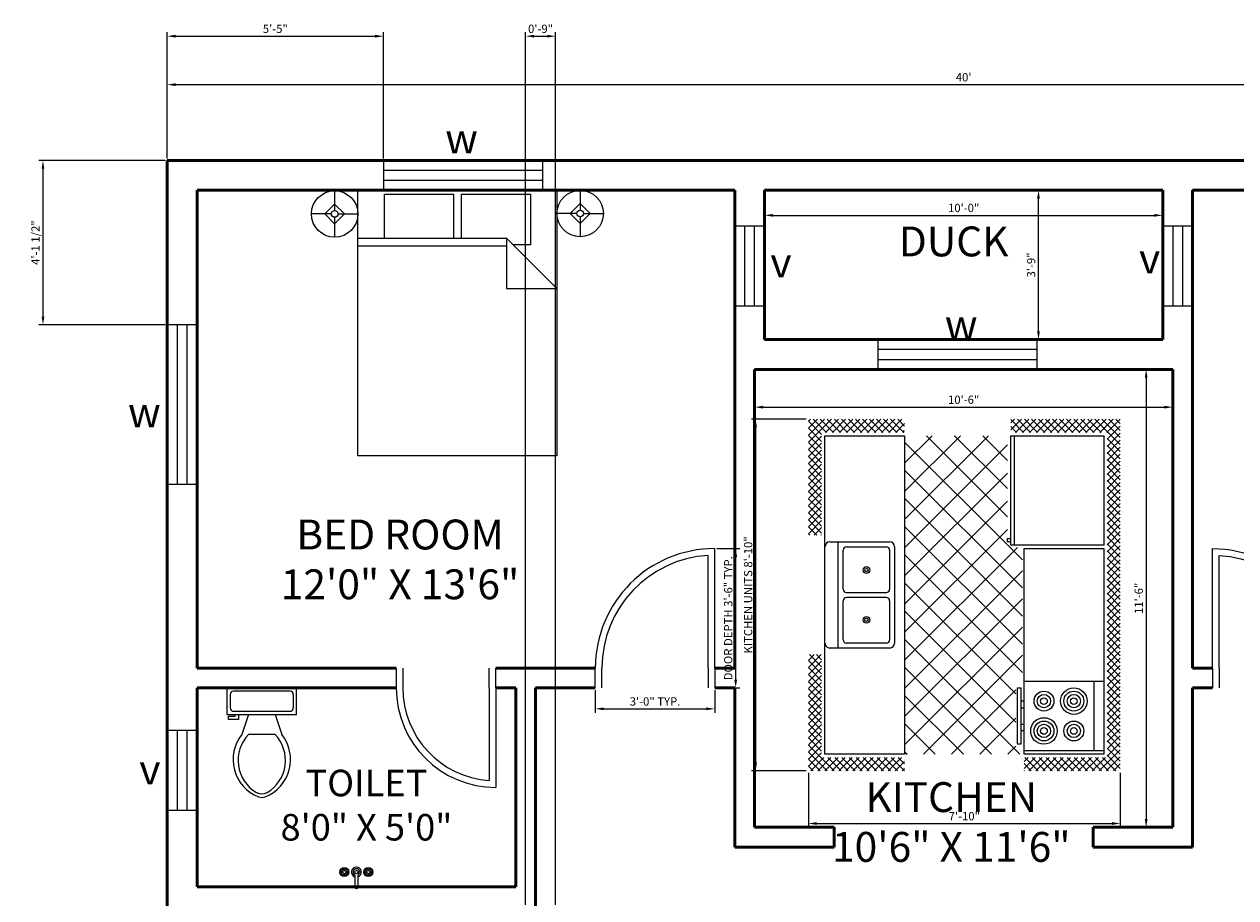
# Model space of a CAD drawing. Units: inches. Extents: x 1776 to 2338, y 1299 to 2099.
# Tile 3 of 4: x 1776 to 2141, y 1836 to 2099. Entities that reach past the tile are written whole.
import ezdxf

# ---------------------------------------------------------------- set-up
doc = ezdxf.new("R2010")
doc.units = ezdxf.units.IN
for name, color, linetype, lineweight in [('A-ANNO-DIMS', 2, 'Continuous', 18), ('A-ANNO-TEXT', 7, 'Continuous', 18), ('A-AREA-IDEN', 7, 'Continuous', 25), ('A-DOOR', 4, 'Continuous', 25), ('A-FLOR-FIXT', 9, 'Continuous', 18), ('A-FURN', 8, 'Continuous', 18), ('A-GLAZ', 4, 'Continuous', 18), ('A-WALL', 7, 'Continuous', 50), ('E-LITE', 9, 'Continuous', 18)]:
    doc.layers.add(name, color=color, linetype=linetype, lineweight=lineweight)
doc.styles.get("Standard").update_dxf_attribs({"font": 'arial.ttf'})
doc.dimstyles.new('ISO-25', dxfattribs={"dimtxt": 2.5, "dimasz": 2.5, "dimexe": 1.25, "dimexo": 0.625, "dimtad": 1, "dimdec": 0, "dimlunit": 3, "dimtxsty": 'Standard', "dimcen": 2.5, "dimadec": 0, "dimazin": 0, "dimtfac": 1, "dimtdec": 0, "dimtmove": 0, "dimatfit": 3, "dimfxl": 1, "dimarcsym": 0})

# ---------------------------------------------------------------- blocks, each defined once
blk = doc.blocks.new('Kitchen Layout - 7 x 8 ft')
for p, q in [((-5, 81.32), (2.68, 89)), ((-5, 83.44), (0.56, 89)), ((-5, 85.56), (-1.56, 89)), ((-5, 87.68), (-3.68, 89)), ((-1, 84.97), (-5, 88.97)), ((1.09, 85), (-2.91, 89)), ((3.21, 85), (-0.79, 89)), ((0.81, 85), (4.81, 89)), ((5.34, 85), (1.34, 89)), ((2.93, 85), (6.93, 89)), ((7.46, 85), (3.46, 89)), ((5.05, 85), (9.05, 89)), ((9.58, 85), (5.58, 89)), ((7.17, 85), (11.17, 89)), ((11.7, 85), (7.7, 89)), ((9.29, 85), (13.29, 89)), ((13.82, 85), (9.82, 89)), ((11.41, 85), (15.41, 89)), ((15.94, 85), (11.94, 89)), ((13.53, 85), (17.53, 89)), ((18.06, 85), (14.06, 89)), ((15.65, 85), (19.65, 89)), ((20.18, 85), (16.18, 89)), ((17.78, 85), (21.78, 89)), ((22.31, 85), (18.31, 89)), ((19.9, 85), (23.9, 89)), ((24.43, 85), (20.43, 89)), ((22.02, 85), (26.02, 89)), ((26.55, 85), (22.55, 89)), ((24.14, 85), (28.14, 89)), ((28.67, 85), (24.67, 89)), ((26.26, 85), (30.26, 89)), ((30.79, 85), (26.79, 89)), ((28.38, 85), (32.38, 89)), ((32.91, 85), (28.91, 89)), ((30.5, 85), (34.5, 89)), ((35.03, 85), (31.03, 89)), ((32.63, 85), (36.63, 89)), ((37.16, 85), (33.16, 89)), ((34.75, 85), (38.75, 89)), ((39.28, 85), (35.28, 89)), ((36.87, 85), (40.87, 89)), ((41.4, 85), (37.4, 89)), ((38.99, 85), (42.99, 89)), ((43.52, 85), (39.52, 89)), ((41.11, 85), (45.11, 89)), ((45.64, 85), (41.64, 89)), ((43.23, 85), (47.23, 89)), ((47.76, 85), (43.76, 89)), ((45.35, 85), (49.35, 89)), ((49.88, 85), (45.88, 89)), ((47.47, 85), (51.47, 89)), ((52, 85), (48, 89)), ((49.6, 85), (53.6, 89)), ((54.13, 85), (50.13, 89)), ((51.72, 85), (55.72, 89)), ((56.25, 85), (52.25, 89)), ((53.84, 85), (57.84, 89)), ((58.37, 85), (54.37, 89)), ((55.96, 85), (59.96, 89)), ((60.49, 85), (56.49, 89)), ((58.08, 85), (62.08, 89)), ((62.61, 85), (58.61, 89)), ((60.2, 85), (64.2, 89)), ((64.73, 85), (60.73, 89)), ((62.32, 85), (66.32, 89)), ((66.85, 85), (62.85, 89)), ((64.45, 85), (68.45, 89)), ((68.97, 85), (64.97, 89)), ((66.57, 85), (70.57, 89)), ((71.1, 85), (67.1, 89)), ((68.69, 85), (72.69, 89)), ((73.22, 85), (69.22, 89)), ((70.81, 85), (74.81, 89)), ((75.34, 85), (71.34, 89)), ((72.93, 85), (76.93, 89)), ((77.46, 85), (73.46, 89)), ((75.05, 85), (79.05, 89)), ((79.58, 85), (75.58, 89)), ((77.17, 85), (81.17, 89)), ((81.7, 85), (77.7, 89)), ((79.29, 85), (83.29, 89)), ((83.82, 85), (79.82, 89)), ((81.42, 85), (85.42, 89)), ((85.95, 85), (81.95, 89)), ((83.54, 85), (87.54, 89)), ((88.07, 85), (84.07, 89)), ((85.66, 85), (89.66, 89)), ((90.19, 85), (86.19, 89)), ((87.78, 85), (91.78, 89)), ((92.31, 85), (88.31, 89)), ((89.9, 85), (93.9, 89)), ((94.43, 85), (90.43, 89)), ((92.02, 85), (96.02, 89)), ((96.55, 85), (92.55, 89)), ((94.14, 85), (98.14, 89)), ((101, 82.67), (94.67, 89)), ((96.27, 85), (100.27, 89)), ((101, 84.79), (96.79, 89)), ((101, 86.92), (98.92, 89)), ((-1, 82.85), (-5, 86.85)), ((-1, 80.73), (-5, 84.73)), ((34, 84), (96, 84)), ((34, 60), (34, 84)), ((96, 84), (96, 60)), ((97, 83.61), (101, 87.61)), ((97, 81.49), (101, 85.49)), ((101, 80.55), (97, 84.55)), ((-5, 79.19), (-1, 83.19)), ((-1, 78.61), (-5, 82.61)), ((-5, 77.07), (-1, 81.07)), ((-1, 76.49), (-5, 80.49)), ((74, 81), (95, 81)), ((97, 79.37), (101, 83.37)), ((101, 78.43), (97, 82.43)), ((97, 77.25), (101, 81.25)), ((-5, 74.95), (-1, 78.95)), ((-1, 74.36), (-5, 78.36)), ((-5, 72.83), (-1, 76.83)), ((101, 76.31), (97, 80.31)), ((97, 75.13), (101, 79.13)), ((101, 74.19), (97, 78.19)), ((97, 73.01), (101, 77.01)), ((-1, 72.24), (-5, 76.24)), ((-5, 70.71), (-1, 74.71)), ((-1, 70.12), (-5, 74.12)), ((101, 72.07), (97, 76.07)), ((97, 70.89), (101, 74.89)), ((101, 69.95), (97, 73.95)), ((-5, 68.59), (-1, 72.59)), ((-1, 68), (-5, 72)), ((-5, 66.47), (-1, 70.47)), ((-1, 65.88), (-5, 69.88)), ((97, 68.76), (101, 72.76)), ((101, 67.82), (97, 71.82)), ((97, 66.64), (101, 70.64)), ((101, 65.7), (97, 69.7)), ((-5, 64.35), (-1, 68.35)), ((-1, 63.76), (-5, 67.76)), ((-5, 62.22), (-1, 66.22)), ((97, 64.52), (101, 68.52)), ((101, 63.58), (97, 67.58)), ((97, 62.4), (101, 66.4)), ((-1, 61.64), (-5, 65.64)), ((-5, 60.1), (-1, 64.1)), ((-1, 59.52), (-5, 63.52)), ((101, 61.46), (97, 65.46)), ((97, 60.28), (101, 64.28)), ((100.34, 60), (97, 63.34)), ((98.84, 60), (101, 62.16)), ((-5, 57.98), (-1, 61.98)), ((-1, 57.39), (-5, 61.39)), ((-1.73, 56), (-5, 59.27)), ((-4.86, 56), (-1, 59.86)), ((10.4, 24), (45.9, 59.5)), ((18.88, 24), (54.38, 59.5)), ((27.37, 24), (62.87, 59.5)), ((33.03, 55.11), (37.41, 59.5)), ((96, 60), (34, 60)), ((35.85, 24), (71.35, 59.5)), ((76.2, 24), (40.7, 59.5)), ((84.68, 24), (49.18, 59.5)), ((93.17, 24), (57.67, 59.5)), ((61.31, 24), (96, 58.69)), ((96, 29.65), (66.15, 59.5)), ((80, 60), (80, 59)), ((82, 59), (82, 60)), ((87, 59), (87, 60)), ((89, 60), (89, 59)), ((98.22, 60), (97, 61.22)), ((100.96, 60), (101, 60.04)), ((-3.85, 56), (-5, 57.15)), ((-2.74, 56), (-1, 57.74)), ((0, 57), (33, 57)), ((0, 30.57), (24.43, 55)), ((0, 39.06), (15.94, 55)), ((0, 47.54), (7.46, 55)), ((1.91, 24), (32.91, 55)), ((33.77, 24), (2.77, 55)), ((42.26, 24), (11.26, 55)), ((50.74, 24), (19.74, 55)), ((59.23, 24), (28.23, 55)), ((31, 55), (31, 56)), ((32, 55), (31, 55)), ((32, 56), (32, 55)), ((67.71, 24), (33.68, 58.04)), ((44.34, 24), (77.84, 57.5)), ((52.82, 24), (86.32, 57.5)), ((96, 38.14), (76.64, 57.5)), ((96, 46.63), (85.13, 57.5)), ((96, 55.11), (93.57, 57.54)), ((25.29, 24), (0, 49.29)), ((69.79, 24), (96, 50.21)), ((16.8, 24), (0, 40.8)), ((78.28, 24), (96, 41.72)), ((86.76, 24), (96, 33.24)), ((8.32, 24), (0, 32.32)), ((-5, 21.92), (-2.92, 24)), ((-5, 19.8), (-1, 23.8)), ((-1, 19.21), (-5, 23.21)), ((-1, 21.33), (-3.67, 24)), ((-1, 23.45), (-1.55, 24)), ((0, 24), (96, 24)), ((0, 0), (0, 24)), ((95.25, 24), (96, 24.75)), ((96, 24), (96, 0)), ((97, 22.1), (98.9, 24)), ((97, 19.97), (101, 23.97)), ((101, 19.03), (97, 23.03)), ((101, 21.16), (98.16, 24)), ((101, 23.28), (100.28, 24)), ((-5, 17.68), (-1, 21.68)), ((-1, 17.09), (-5, 21.09)), ((-5, 15.55), (-1, 19.55)), ((-1, 14.97), (-5, 18.97)), ((47.25, 6.5), (47.25, 18.5)), ((48.75, 18.5), (48.75, 6.5)), ((97, 17.85), (101, 21.85)), ((101, 16.91), (97, 20.91)), ((97, 15.73), (101, 19.73)), ((101, 14.79), (97, 18.79)), ((-5, 13.43), (-1, 17.43)), ((-1, 12.85), (-5, 16.85)), ((-5, 11.31), (-1, 15.31)), ((-1, 10.73), (-5, 14.73)), ((97, 13.61), (101, 17.61)), ((101, 12.67), (97, 16.67)), ((97, 11.49), (101, 15.49)), ((-5, 9.19), (-1, 13.19)), ((-1, 8.6), (-5, 12.6)), ((-5, 7.07), (-1, 11.07)), ((101, 10.55), (97, 14.55)), ((97, 9.37), (101, 13.37)), ((101, 8.43), (97, 12.43)), ((97, 7.25), (101, 11.25)), ((-1, 6.48), (-5, 10.48)), ((-5, 4.95), (-1, 8.95)), ((-1, 4.36), (-5, 8.36)), ((101, 6.31), (97, 10.31)), ((97, 5.12), (101, 9.12)), ((101, 4.18), (97, 8.18)), ((-5, 2.83), (-1, 6.83)), ((-1, 2.24), (-5, 6.24)), ((-5, 0.71), (-1, 4.71)), ((-1, 0.12), (-5, 4.12)), ((64, 4), (32, 4)), ((97, 3), (101, 7)), ((101, 2.06), (97, 6.06)), ((97, 0.88), (101, 4.88)), ((101, -0.06), (97, 3.94)), ((-5, -1.42), (-1, 2.58)), ((2, -5), (-5, 2)), ((-5, -3.54), (-1, 0.46)), ((96, 0), (0, 0)), ((93.24, -5), (101, 2.76)), ((95.36, -5), (101, 0.64)), ((101, -2.18), (97, 1.82)), ((-0.12, -5), (-5, -0.12)), ((-2.25, -5), (-5, -2.25)), ((-4.34, -5), (-0.34, -1)), ((-2.22, -5), (1.78, -1)), ((-0.1, -5), (3.9, -1)), ((4.12, -5), (0.12, -1)), ((2.02, -5), (6.02, -1)), ((6.24, -5), (2.24, -1)), ((4.14, -5), (8.14, -1)), ((8.36, -5), (4.36, -1)), ((6.27, -5), (10.27, -1)), ((10.48, -5), (6.48, -1)), ((8.39, -5), (12.39, -1)), ((12.6, -5), (8.6, -1)), ((10.51, -5), (14.51, -1)), ((14.73, -5), (10.73, -1)), ((12.63, -5), (16.63, -1)), ((16.85, -5), (12.85, -1)), ((14.75, -5), (18.75, -1)), ((18.97, -5), (14.97, -1)), ((16.87, -5), (20.87, -1)), ((21.09, -5), (17.09, -1)), ((18.99, -5), (22.99, -1)), ((23.21, -5), (19.21, -1)), ((21.11, -5), (25.11, -1)), ((25.33, -5), (21.33, -1)), ((23.24, -5), (27.24, -1)), ((27.45, -5), (23.45, -1)), ((25.36, -5), (29.36, -1)), ((29.57, -5), (25.57, -1)), ((27.48, -5), (30, -2.48)), ((30, -3.3), (27.7, -1)), ((30, -1.18), (29.82, -1)), ((66, -2.54), (67.54, -1)), ((66, -4.66), (69.66, -1)), ((69.88, -5), (66, -1.12)), ((67.76, -5), (66, -3.24)), ((67.78, -5), (71.78, -1)), ((72, -5), (68, -1)), ((69.9, -5), (73.9, -1)), ((74.12, -5), (70.12, -1)), ((72.03, -5), (76.03, -1)), ((76.24, -5), (72.24, -1)), ((74.15, -5), (78.15, -1)), ((78.36, -5), (74.36, -1)), ((76.27, -5), (80.27, -1)), ((80.49, -5), (76.49, -1)), ((78.39, -5), (82.39, -1)), ((82.61, -5), (78.61, -1)), ((80.51, -5), (84.51, -1)), ((84.73, -5), (80.73, -1)), ((82.63, -5), (86.63, -1)), ((86.85, -5), (82.85, -1)), ((84.75, -5), (88.75, -1)), ((88.97, -5), (84.97, -1)), ((86.88, -5), (90.88, -1)), ((91.09, -5), (87.09, -1)), ((89, -5), (93, -1)), ((93.21, -5), (89.21, -1)), ((91.12, -5), (95.12, -1)), ((95.34, -5), (91.34, -1)), ((97.46, -5), (93.46, -1)), ((99.58, -5), (95.58, -1)), ((101, -4.3), (97, -0.3)), ((97.48, -5), (101, -1.48)), ((99.6, -5), (101, -3.6)), ((-4.37, -5), (-5, -4.37)), ((29.6, -5), (30, -4.6))]:
    blk.add_line(p, q)
for points in [[(0, 56), (0, 84), (33, 84), (33, 56)], [(74, 60), (74, 84), (95, 84), (95, 60)], [(76, 58), (76, 59), (93, 59), (93, 58)]]:
    blk.add_lwpolyline(points, close=True)
for points in [[(32, 1.5), (32, 19.5)], [(33.5, 21), (62.5, 21)], [(33.5, 6.5), (33.5, 18.5)], [(34.5, 19.5), (46.25, 19.5)], [(49.75, 19.5), (61.5, 19.5)], [(62.5, 18.5), (62.5, 6.5)], [(64, 19.5), (64, 1.5)], [(46.25, 5.5), (34.5, 5.5)], [(61.5, 5.5), (49.75, 5.5)], [(62.5, 0), (33.5, 0)]]:
    blk.add_lwpolyline(points)
for centre, radius in [((80, 75), 4), ((80, 75), 3), ((80, 75), 2), ((89, 75), 3), ((89, 75), 2), ((80, 75), 1), ((89, 75), 1), ((89, 66), 4), ((80, 66), 3), ((80, 66), 2), ((80, 66), 1), ((89, 66), 3), ((89, 66), 2), ((89, 66), 1), ((40.5, 12.5), 1), ((40.5, 12.5), 0.5), ((55.5, 12.5), 1), ((55.5, 12.5), 0.5)]:
    blk.add_circle(centre, radius)
for centre, radius, start, end in [((33.5, 19.5), 1.5, 90, 180), ((34.5, 18.5), 1, 90, 180), ((46.25, 18.5), 1, 0, 90), ((49.75, 18.5), 1, 90, 180), ((61.5, 18.5), 1, 0, 90), ((62.5, 19.5), 1.5, 0, 90), ((34.5, 6.5), 1, 180, 270), ((46.25, 6.5), 1, 270, 0), ((49.75, 6.5), 1, 180, 270), ((61.5, 6.5), 1, 270, 0), ((33.5, 1.5), 1.5, 180, 270), ((62.5, 1.5), 1.5, 270, 0)]:
    blk.add_arc(centre, radius, start, end)
blk = doc.blocks.new('Bed - Queen')
for p, q in [((0, -80.00003), (0, 0)), ((0, 0), (59.99999, 0)), ((59.99999, 0), (59.99999, -80.00003)), ((7.99999, -1.2), (28.79998, -1.2)), ((7.99999, -14.4), (7.99999, -1.2)), ((28.79998, -1.2), (28.79998, -14.4)), ((31.19999, -1.2), (51.99999, -1.2)), ((31.19999, -14.4), (31.19999, -1.2)), ((51.99999, -1.2), (51.99999, -16.4)), ((0, -14.4), (44.8, -14.4)), ((59.99999, -29.6), (44.8, -14.4)), ((44.8, -14.4), (44.8, -29.6)), ((44.8, -16.8), (0, -16.8)), ((51.99999, -16.4), (46.79936, -16.4)), ((44.8, -29.6), (59.99999, -29.6)), ((59.99999, -80.00003), (0, -80.00003))]:
    blk.add_line(p, q)
blk = doc.blocks.new('Lamp - Table')
for p, q in [((0, 7), (0, 1)), ((-1, 0), (-7, 0)), ((0, 3), (-3, 0)), ((-3, 0), (0, -3)), ((3, 0), (0, 3)), ((0, -3), (3, 0)), ((1, 0), (7, 0)), ((0, -1), (0, -7))]:
    blk.add_line(p, q)
for radius in [7, 1]:
    blk.add_circle((0, 0), radius)
blk = doc.blocks.new('Toilet - top')
for p, q in [((9.5, -6), (9.5, -2)), ((-10, -8.5), (-8, -8.5)), ((-10, -9.5), (-10, -8.5)), ((-7, -9.5), (-10, -9.5)), ((-8, -8.5), (-8, -8)), ((-7, -8), (-7, -9.5)), ((-4, -8), (-6, -14)), ((4, -8), (6, -14)), ((4, -14), (-4, -14))]:
    blk.add_line(p, q)
blk.add_lwpolyline([(10.5, -8), (10.5, 0), (-10.5, 0), (-10.5, -8)], close=True)
for points in [[(-9.5, -2), (-9.5, -6)], [(8.5, -1), (-8.5, -1)], [(-8.5, -7), (8.5, -7)]]:
    blk.add_lwpolyline(points)
for centre, radius, start, end in [((-8.62, -1.88), 0.884, 81.8699, 188.1301), ((8.62, -1.88), 0.884, 351.8699, 98.1301), ((-8.62, -6.12), 0.884, 171.8699, 278.1301), ((8.62, -6.12), 0.884, 261.8699, 8.1301), ((3.52, -21.58), 12.17, 141.4691, 247.9714), ((4.2, -21.82), 11.33, 136.3677, 238.9468), ((-3.52, -21.58), 12.17, 292.0284, 38.5307), ((-4.2, -21.82), 11.33, 301.053, 43.6321), ((0, -27.88), 4, 245.7318, 294.2682), ((0, -29), 4, 254.8605, 285.1395)]:
    blk.add_arc(centre, radius, start, end)
blk = doc.blocks.new('Faucet - Bathroom top')
for p, q in [((-4.107, 0.125), (-4.375, 0.125)), ((-3.75, 0.4788), (-3.75, 0.75)), ((-3.5, 0.482), (-3.5, 0.75)), ((-3.1461, 0.125), (-2.875, 0.125)), ((3.143, 0.125), (2.875, 0.125)), ((3.5, 0.4788), (3.5, 0.75)), ((3.75, 0.482), (3.75, 0.75)), ((4.1039, 0.125), (4.375, 0.125)), ((-4.1039, -0.125), (-4.375, -0.125)), ((-3.75, -0.4821), (-3.75, -0.75)), ((-3.5, -0.4789), (-3.5, -0.75)), ((-3.143, -0.125), (-2.875, -0.125)), ((-0.5, -0.8639), (-0.5, -4.5)), ((0.5, -4.5), (0.5, -0.8631)), ((3.1461, -0.125), (2.875, -0.125)), ((3.5, -0.4821), (3.5, -0.75)), ((3.75, -0.4789), (3.75, -0.75)), ((4.107, -0.125), (4.375, -0.125))]:
    blk.add_line(p, q)
for centre, radius in [((-3.625, 0), 1.375), ((-4.625, 0), 0.2795), ((-3.625, 0), 0.5), ((-3.625, 1), 0.2795), ((-2.625, 0), 0.2795), ((0, 0), 0.5), ((3.625, 0), 1.375), ((2.625, 0), 0.2795), ((3.625, 0), 0.5), ((3.625, 1), 0.2795), ((4.625, 0), 0.2795), ((-3.625, -1), 0.2795), ((3.625, -1), 0.2795)]:
    blk.add_circle(centre, radius)
for centre, radius, start, end in [((-3.625, 0), 1, 105.2407, 164.2093), ((-3.625, 0), 1, 16.44125, 74.07887), ((0, 0), 1.5, 289.6514, 250.3603), ((0, 0), 1, 300.3431, 239.7554), ((3.625, 0), 1, 106.12, 164.0884), ((3.625, 0), 1, 16.23422, 73.90469), ((-3.625, 0), 1, 196.2342, 253.9047), ((-3.625, 0), 1, 286.12, 344.0884), ((3.625, 0), 1, 196.4413, 254.0789), ((3.625, 0), 1, 285.2407, 344.2093), ((0, -4.5), 0.5, 180, 0)]:
    blk.add_arc(centre, radius, start, end)
blk = doc.blocks.new('*D9')
at = {"layer": 'A-ANNO-DIMS', "color": 0, "lineweight": -2, "transparency": 16777216}
for p, q in [((1995.74, 1994.59), (1995.74, 1982.6)), ((2121.74, 1994.59), (2121.74, 1982.6)), ((1998.24, 1983.85), (2119.24, 1983.85))]:
    blk.add_line(p, q, dxfattribs=at)
at = {"layer": 'A-ANNO-DIMS', "color": 0, "transparency": 16777216}
for points in [[(1998.24, 1984.27), (1998.24, 1983.44), (1995.74, 1983.85)], [(2119.24, 1984.27), (2119.24, 1983.44), (2121.74, 1983.85)]]:
    blk.add_solid(points, dxfattribs=at)
at = {"layer": 'Defpoints', "color": 0, "transparency": 16777216}
for p in [(1995.74, 1995.22), (2121.74, 1995.22), (2121.74, 1983.85)]:
    blk.add_point(p, dxfattribs=at)
at = {"layer": 'A-ANNO-DIMS', "color": 0, "transparency": 16777216, "insert": (2058.74, 1985.76), "char_height": 2.5, "attachment_point": 5}
blk.add_mtext('10\'-6"', dxfattribs=at)
blk = doc.blocks.new('*D10')
at = {"layer": 'A-ANNO-DIMS', "color": 0, "lineweight": -2, "transparency": 16777216}
for p, q in [((2121.11, 1995.22), (2112.49, 1995.22)), ((2113.74, 1992.72), (2113.74, 1859.72)), ((2121.11, 1857.22), (2112.49, 1857.22))]:
    blk.add_line(p, q, dxfattribs=at)
at = {"layer": 'A-ANNO-DIMS', "color": 0, "transparency": 16777216}
for points in [[(2113.32, 1992.72), (2114.15, 1992.72), (2113.74, 1995.22)], [(2113.32, 1859.72), (2114.15, 1859.72), (2113.74, 1857.22)]]:
    blk.add_solid(points, dxfattribs=at)
at = {"layer": 'Defpoints', "color": 0, "transparency": 16777216}
for p in [(2121.74, 1995.22), (2113.74, 1857.22), (2121.74, 1857.22)]:
    blk.add_point(p, dxfattribs=at)
at = {"layer": 'A-ANNO-DIMS', "color": 0, "transparency": 16777216, "insert": (2111.83, 1926.22), "char_height": 2.5, "attachment_point": 5, "rotation": 90}
blk.add_mtext('11\'-6"', dxfattribs=at)
blk = doc.blocks.new('*D12')
at = {"layer": 'A-ANNO-DIMS', "color": 0, "lineweight": -2, "transparency": 16777216}
for p, q in [((1818.74, 2058.84), (1818.74, 2082.32)), ((1821.24, 2081.07), (2296.24, 2081.07)), ((2298.74, 2058.84), (2298.74, 2082.32))]:
    blk.add_line(p, q, dxfattribs=at)
at = {"layer": 'A-ANNO-DIMS', "color": 0, "transparency": 16777216}
for points in [[(1821.24, 2081.49), (1821.24, 2080.65), (1818.74, 2081.07)], [(2296.24, 2081.49), (2296.24, 2080.65), (2298.74, 2081.07)]]:
    blk.add_solid(points, dxfattribs=at)
at = {"layer": 'Defpoints', "color": 0, "transparency": 16777216}
for p in [(2298.74, 2081.07), (1818.74, 2058.22), (2298.74, 2058.22)]:
    blk.add_point(p, dxfattribs=at)
at = {"layer": 'A-ANNO-DIMS', "color": 0, "transparency": 16777216, "insert": (2058.74, 2082.97), "char_height": 2.5, "attachment_point": 5}
blk.add_mtext("40'", dxfattribs=at)
blk = doc.blocks.new('WIN-48IN')
for p, q in [((48, 9), (0, 9)), ((0, 9), (0, 0)), ((48, 0), (48, 9)), ((48, 6), (0, 6)), ((0, 3), (48, 3)), ((0, 0), (48, 0))]:
    blk.add_line(p, q)
blk = doc.blocks.new('VENT-24IN')
for p, q in [((9, 24), (0, 24)), ((0, 24), (0, 0)), ((3, 24), (3, 0)), ((6, 0), (6, 24)), ((9, 0), (9, 24)), ((0, 0), (9, 0))]:
    blk.add_line(p, q)
blk = doc.blocks.new('DOOR-36IN')
for p, q in [((36, 6), (36, 42)), ((34, 6), (34, 39.94)), ((0, 0), (0, 6)), ((2, 0), (2, 6)), ((34, 6), (34, 0)), ((36, 6), (36, 0))]:
    blk.add_line(p, q)
for radius, start in [(36, 90), (34, 93.3723)]:
    blk.add_arc((36, 6), radius, start, 180)
blk = doc.blocks.new('DOOR-30IN')
for p, q in [((0, 36), (0, 30)), ((2, 36), (2, 30)), ((28, 30), (28, 36)), ((30, 30), (30, 36)), ((28, 30), (28, 2.07)), ((30, 30), (30, 0))]:
    blk.add_line(p, q)
for radius, end in [(30, 270), (28, 265.904)]:
    blk.add_arc((30, 30), radius, 180, end)
blk = doc.blocks.new('*D30')
at = {"layer": 'A-ANNO-DIMS', "color": 0, "lineweight": -2, "transparency": 16777216}
for p, q in [((1984.36, 1941.22), (1991.29, 1941.22)), ((1990.04, 1901.72), (1990.04, 1938.72)), ((1984.36, 1899.22), (1991.29, 1899.22))]:
    blk.add_line(p, q, dxfattribs=at)
at = {"layer": 'A-ANNO-DIMS', "color": 0, "transparency": 16777216}
for points in [[(1989.62, 1938.72), (1990.46, 1938.72), (1990.04, 1941.22)], [(1989.62, 1901.72), (1990.46, 1901.72), (1990.04, 1899.22)]]:
    blk.add_solid(points, dxfattribs=at)
at = {"layer": 'Defpoints', "color": 0, "transparency": 16777216}
for p in [(1983.74, 1941.22), (1990.04, 1941.22), (1983.74, 1899.22)]:
    blk.add_point(p, dxfattribs=at)
at = {"layer": 'A-ANNO-DIMS', "color": 0, "transparency": 16777216, "insert": (1988.12, 1920.22), "char_height": 2.5, "attachment_point": 5, "rotation": 90}
blk.add_mtext('DOOR DEPTH 3\'-6" TYP.', dxfattribs=at)
blk = doc.blocks.new('*D31')
at = {"layer": 'A-ANNO-DIMS', "color": 0, "lineweight": -2, "transparency": 16777216}
for p, q in [((1947.74, 1898.59), (1947.74, 1891.67)), ((1983.74, 1898.59), (1983.74, 1891.67)), ((1950.24, 1892.92), (1981.24, 1892.92))]:
    blk.add_line(p, q, dxfattribs=at)
at = {"layer": 'A-ANNO-DIMS', "color": 0, "transparency": 16777216}
for points in [[(1950.24, 1893.34), (1950.24, 1892.5), (1947.74, 1892.92)], [(1981.24, 1893.34), (1981.24, 1892.5), (1983.74, 1892.92)]]:
    blk.add_solid(points, dxfattribs=at)
at = {"layer": 'Defpoints', "color": 0, "transparency": 16777216}
for p in [(1947.74, 1899.22), (1983.74, 1899.22), (1983.74, 1892.92)]:
    blk.add_point(p, dxfattribs=at)
at = {"layer": 'A-ANNO-DIMS', "color": 0, "transparency": 16777216, "insert": (1965.74, 1894.82), "char_height": 2.5, "attachment_point": 5}
blk.add_mtext('3\'-0" TYP.', dxfattribs=at)
blk = doc.blocks.new('*D40')
at = {"layer": 'A-ANNO-DIMS', "color": 0, "lineweight": -2, "transparency": 16777216}
for p, q in [((2011.31, 1980.25), (1994.79, 1980.25)), ((1996.04, 1977.75), (1996.04, 1876.75)), ((2011.31, 1874.25), (1994.79, 1874.25))]:
    blk.add_line(p, q, dxfattribs=at)
at = {"layer": 'A-ANNO-DIMS', "color": 0, "transparency": 16777216}
for points in [[(1995.62, 1977.75), (1996.45, 1977.75), (1996.04, 1980.25)], [(1995.62, 1876.75), (1996.45, 1876.75), (1996.04, 1874.25)]]:
    blk.add_solid(points, dxfattribs=at)
at = {"layer": 'Defpoints', "color": 0, "transparency": 16777216}
for p in [(2011.94, 1980.25), (1996.04, 1874.25), (2011.94, 1874.25)]:
    blk.add_point(p, dxfattribs=at)
at = {"layer": 'A-ANNO-DIMS', "color": 0, "transparency": 16777216, "insert": (1994.12, 1927.25), "char_height": 2.5, "attachment_point": 5, "rotation": 90}
blk.add_mtext('KITCHEN UNITS 8\'-10"', dxfattribs=at)
blk = doc.blocks.new('*D41')
at = {"layer": 'A-ANNO-DIMS', "color": 0, "lineweight": -2, "transparency": 16777216}
for p, q in [((2011.94, 1873.62), (2011.94, 1857.1)), ((2105.94, 1873.62), (2105.94, 1857.1)), ((2014.44, 1858.35), (2103.44, 1858.35))]:
    blk.add_line(p, q, dxfattribs=at)
at = {"layer": 'A-ANNO-DIMS', "color": 0, "transparency": 16777216}
for points in [[(2014.44, 1858.77), (2014.44, 1857.93), (2011.94, 1858.35)], [(2103.44, 1858.77), (2103.44, 1857.93), (2105.94, 1858.35)]]:
    blk.add_solid(points, dxfattribs=at)
at = {"layer": 'Defpoints', "color": 0, "transparency": 16777216}
for p in [(2011.94, 1874.25), (2105.94, 1874.25), (2105.94, 1858.35)]:
    blk.add_point(p, dxfattribs=at)
at = {"layer": 'A-ANNO-DIMS', "color": 0, "transparency": 16777216, "insert": (2058.94, 1860.25), "char_height": 2.5, "attachment_point": 5}
blk.add_mtext('7\'-10"', dxfattribs=at)
blk = doc.blocks.new('*D45')
at = {"layer": 'A-ANNO-DIMS', "color": 0, "lineweight": -2, "transparency": 16777216}
for p, q in [((1998.74, 2004.84), (1998.74, 2042.92)), ((2001.24, 2041.67), (2116.24, 2041.67)), ((2118.74, 2004.84), (2118.74, 2042.92))]:
    blk.add_line(p, q, dxfattribs=at)
at = {"layer": 'A-ANNO-DIMS', "color": 0, "transparency": 16777216}
for points in [[(2001.24, 2042.09), (2001.24, 2041.25), (1998.74, 2041.67)], [(2116.24, 2042.09), (2116.24, 2041.25), (2118.74, 2041.67)]]:
    blk.add_solid(points, dxfattribs=at)
at = {"layer": 'Defpoints', "color": 0, "transparency": 16777216}
for p in [(2118.74, 2041.67), (1998.74, 2004.22), (2118.74, 2004.22)]:
    blk.add_point(p, dxfattribs=at)
at = {"layer": 'A-ANNO-DIMS', "color": 0, "transparency": 16777216, "insert": (2058.74, 2043.57), "char_height": 2.5, "attachment_point": 5}
blk.add_mtext('10\'-0"', dxfattribs=at)
blk = doc.blocks.new('*D46')
at = {"layer": 'A-ANNO-DIMS', "color": 0, "lineweight": -2, "transparency": 16777216}
for p, q in [((2118.11, 2049.22), (2080.04, 2049.22)), ((2081.29, 2006.72), (2081.29, 2046.72)), ((2118.11, 2004.22), (2080.04, 2004.22))]:
    blk.add_line(p, q, dxfattribs=at)
at = {"layer": 'A-ANNO-DIMS', "color": 0, "transparency": 16777216}
for points in [[(2080.87, 2046.72), (2081.71, 2046.72), (2081.29, 2049.22)], [(2080.87, 2006.72), (2081.71, 2006.72), (2081.29, 2004.22)]]:
    blk.add_solid(points, dxfattribs=at)
at = {"layer": 'Defpoints', "color": 0, "transparency": 16777216}
for p in [(2081.29, 2049.22), (2118.74, 2049.22), (2118.74, 2004.22)]:
    blk.add_point(p, dxfattribs=at)
at = {"layer": 'A-ANNO-DIMS', "color": 0, "transparency": 16777216, "insert": (2079.39, 2026.72), "char_height": 2.5, "attachment_point": 5, "rotation": 90}
blk.add_mtext('3\'-9"', dxfattribs=at)
blk = doc.blocks.new('*D49')
at = {"layer": 'A-ANNO-DIMS', "color": 0, "lineweight": -2, "transparency": 16777216}
for p, q in [((1926.74, 1833.84), (1926.74, 2096.92)), ((1929.24, 2095.67), (1933.24, 2095.67)), ((1935.74, 1833.84), (1935.74, 2096.92))]:
    blk.add_line(p, q, dxfattribs=at)
at = {"layer": 'A-ANNO-DIMS', "color": 0, "transparency": 16777216}
for points in [[(1929.24, 2096.09), (1929.24, 2095.25), (1926.74, 2095.67)], [(1933.24, 2096.09), (1933.24, 2095.25), (1935.74, 2095.67)]]:
    blk.add_solid(points, dxfattribs=at)
at = {"layer": 'Defpoints', "color": 0, "transparency": 16777216}
for p in [(1935.74, 2095.67), (1926.74, 1833.22), (1935.74, 1833.22)]:
    blk.add_point(p, dxfattribs=at)
at = {"layer": 'A-ANNO-DIMS', "color": 0, "transparency": 16777216, "insert": (1931.24, 2097.57), "char_height": 2.5, "attachment_point": 5}
blk.add_mtext('0\'-9"', dxfattribs=at)
blk = doc.blocks.new('*D51')
at = {"layer": 'A-ANNO-DIMS', "color": 0, "lineweight": -2, "transparency": 16777216}
for p, q in [((1818.74, 2058.84), (1818.74, 2096.92)), ((1821.24, 2095.67), (1881.39, 2095.67)), ((1883.89, 2058.84), (1883.89, 2096.92))]:
    blk.add_line(p, q, dxfattribs=at)
at = {"layer": 'A-ANNO-DIMS', "color": 0, "transparency": 16777216}
for points in [[(1821.24, 2096.09), (1821.24, 2095.25), (1818.74, 2095.67)], [(1881.39, 2096.09), (1881.39, 2095.25), (1883.89, 2095.67)]]:
    blk.add_solid(points, dxfattribs=at)
at = {"layer": 'Defpoints', "color": 0, "transparency": 16777216}
for p in [(1883.89, 2095.67), (1818.74, 2058.22), (1883.89, 2058.22)]:
    blk.add_point(p, dxfattribs=at)
at = {"layer": 'A-ANNO-DIMS', "color": 0, "transparency": 16777216, "insert": (1851.31, 2097.57), "char_height": 2.5, "attachment_point": 5}
blk.add_mtext('5\'-5"', dxfattribs=at)
blk = doc.blocks.new('*D53')
at = {"layer": 'A-ANNO-DIMS', "color": 0, "lineweight": -2, "transparency": 16777216}
for p, q in [((1818.11, 2058.22), (1780.04, 2058.22)), ((1781.29, 2055.72), (1781.29, 2011.17)), ((1818.11, 2008.67), (1780.04, 2008.67))]:
    blk.add_line(p, q, dxfattribs=at)
at = {"layer": 'A-ANNO-DIMS', "color": 0, "transparency": 16777216}
for points in [[(1780.87, 2055.72), (1781.71, 2055.72), (1781.29, 2058.22)], [(1780.87, 2011.17), (1781.71, 2011.17), (1781.29, 2008.67)]]:
    blk.add_solid(points, dxfattribs=at)
at = {"layer": 'Defpoints', "color": 0, "transparency": 16777216}
for p in [(1818.74, 2058.22), (1781.29, 2008.67), (1818.74, 2008.67)]:
    blk.add_point(p, dxfattribs=at)
at = {"layer": 'A-ANNO-DIMS', "color": 0, "transparency": 16777216, "insert": (1779.37, 2033.45), "char_height": 2.5, "attachment_point": 5, "rotation": 90}
blk.add_mtext('4\'-1 1/2"', dxfattribs=at)

msp = doc.modelspace()

# ---------------------------------------------------------------- linework, layer by layer
at = {"layer": 'A-WALL'}
for p, q in [((1818.74, 2058.22), (2298.74, 2058.22)), ((1818.74, 1338.22), (1818.74, 2058.22)), ((1827.74, 2049.22), (1989.74, 2049.22)), ((1827.74, 1905.22), (1827.74, 2049.22)), ((1989.74, 1905.22), (1989.74, 2049.22)), ((1998.74, 2049.22), (2118.74, 2049.22)), ((1998.74, 2004.22), (1998.74, 2049.22)), ((2118.74, 2049.22), (2118.74, 2004.22)), ((2127.74, 2049.22), (2127.74, 1905.22)), ((2127.74, 2049.22), (2289.74, 2049.22)), ((1998.74, 2004.22), (2118.74, 2004.22)), ((1995.74, 1857.22), (1995.74, 1995.22)), ((1995.74, 1995.22), (2121.74, 1995.22)), ((2121.74, 1995.22), (2121.74, 1857.22)), ((1827.74, 1905.22), (1887.74, 1905.22)), ((1917.74, 1905.22), (1947.74, 1905.22)), ((1989.74, 1905.22), (1983.74, 1905.22)), ((1983.74, 1905.22), (1989.74, 1905.22)), ((2127.74, 1905.22), (2133.74, 1905.22)), ((2127.74, 1905.22), (2133.74, 1905.22)), ((1827.74, 1899.22), (1887.74, 1899.22)), ((1827.74, 1839.22), (1827.74, 1899.22)), ((1923.74, 1899.22), (1917.74, 1899.22)), ((1917.74, 1899.22), (1923.74, 1899.22)), ((1923.74, 1839.22), (1923.74, 1899.22)), ((1929.74, 1833.22), (1929.74, 1899.22)), ((1929.74, 1899.22), (1947.74, 1899.22)), ((1983.74, 1899.22), (1989.74, 1899.22)), ((1989.74, 1851.22), (1989.74, 1899.22)), ((2127.74, 1899.22), (2133.74, 1899.22)), ((2127.74, 1899.22), (2127.74, 1851.22)), ((2127.74, 1899.22), (2127.74, 1851.22)), ((1995.74, 1857.22), (2019.74, 1857.22)), ((1995.74, 1857.22), (2019.74, 1857.22)), ((2019.74, 1857.22), (2019.74, 1851.22)), ((2121.74, 1857.22), (2097.74, 1857.22)), ((2097.74, 1857.22), (2097.74, 1851.22)), ((2097.74, 1857.22), (2121.74, 1857.22)), ((1995.74, 1851.22), (1989.74, 1851.22)), ((1995.74, 1851.22), (2019.74, 1851.22)), ((2097.74, 1851.22), (2121.74, 1851.22)), ((2121.74, 1851.22), (2127.74, 1851.22)), ((1827.74, 1839.22), (1923.74, 1839.22))]:
    msp.add_line(p, q, dxfattribs=at)

# ---------------------------------------------------------------- block references
at = {"layer": 'A-DOOR'}
for name, p in [('DOOR-36IN', (1947.74, 1899.22)), ('DOOR-30IN', (1887.74, 1869.22))]:
    msp.add_blockref(name, p, dxfattribs=at)
at = {"layer": 'A-DOOR', "extrusion": (0, 0, -1), "zscale": -1}
msp.add_blockref('DOOR-36IN', (-2169.74, 1899.22), dxfattribs=at)
at = {"layer": 'A-FLOR-FIXT', "rotation": 270}
msp.add_blockref('Kitchen Layout - 7 x 8 ft', (2016.94, 1975.25), dxfattribs=at)
at = {"layer": 'A-FLOR-FIXT'}
for name, p in [('Toilet - top', (1847.24, 1899.22)), ('Faucet - Bathroom top', (1875.74, 1843.72))]:
    msp.add_blockref(name, p, dxfattribs=at)
at = {"layer": 'A-FURN'}
msp.add_blockref('Bed - Queen', (1876.19, 2049.22), dxfattribs=at)
at = {"layer": 'A-GLAZ'}
for p, rotation in [((1931.89, 2058.22), 180), ((1818.74, 2008.67), 269.9999999999979), ((2080.88, 2004.22), 180)]:
    msp.add_blockref('WIN-48IN', p, dxfattribs=dict(at, rotation=rotation))
for p in [(1989.74, 2014.36), (2118.74, 2014.38), (1818.74, 1862.42)]:
    msp.add_blockref('VENT-24IN', p, dxfattribs=at)
at = {"layer": 'E-LITE'}
for p in [(1869.19, 2042.08), (1943.19, 2042.23)]:
    msp.add_blockref('Lamp - Table', p, dxfattribs=at)

# ---------------------------------------------------------------- texts
at = {"layer": 'A-ANNO-TEXT', "char_height": 9, "attachment_point": 1}
for s, heights, insert in [('\\pxqc;w', [0], (1882.32, 2069.37)), ('\\pxqc;v', [47.58], (2089.67, 2033.2)), ('\\pxqc;v', [47.58], (1978.57, 2031.95)), ('\\pxqc;w', [0], (2032.88, 2013.22)), ('\\pxqc;w', [0], (1786.73, 1986.8)), ('\\pxqc;v', [47.58], (1788.4, 1879.14))]:
    msp.add_mtext_dynamic_manual_height_columns(s, width=50.2204, gutter_width=12.5, heights=heights, dxfattribs=dict(at, insert=insert))
at = {"layer": 'A-AREA-IDEN', "attachment_point": 1}
for s, width, insert, char_height in [('\\pxqc;DUCK', 54.1226, (2028.66, 2038.3), 9), ('\\pxqc;BED ROOM \\P12\'0" X 13\'6"', 105.4264, (1836.18, 1949.96), 9), ('\\pxqc;TOILET\\P8\'0" X 5\'0"', 54.6133, (1851.47, 1874.56), 8), ('\\pxqc;KITCHEN\\P10\'6" X 11\'6"', 105.4264, (2002.3, 1870.81), 9)]:
    msp.add_mtext_dynamic_manual_height_columns(s, width=width, gutter_width=12.5, heights=[0], dxfattribs=dict(at, insert=insert, char_height=char_height))

# ---------------------------------------------------------------- dimensions: what is measured, and where the dimension line sits
at = {"layer": 'A-ANNO-DIMS'}
for base, p1, p2, override, picture, middle in [((1883.8886, 2095.6687), (1818.7388, 2058.2187), (1883.8886, 2058.2187), {"dimdec": 1, "dimlfac": 1, "dimrnd": 0, "dimzin": 1, "dimdsep": 46, "dimlunit": 4, "dimfrac": 2}, '*D51', (1851.3137, 2097.5651)), ((1935.74, 2095.67), (1926.74, 1833.22), (1935.74, 1833.22), {"dimdec": 1, "dimlfac": 1, "dimrnd": 0, "dimzin": 1, "dimdsep": 46, "dimlunit": 4, "dimfrac": 2}, '*D49', (1931.24, 2097.57)), ((2298.74, 2081.07), (1818.74, 2058.22), (2298.74, 2058.22), {"dimclrd": 0, "dimclre": 0, "dimclrt": 0}, '*D12', (2058.74, 2082.97)), ((2118.74, 2041.67), (1998.74, 2004.22), (2118.74, 2004.22), {"dimdec": 1, "dimlfac": 1, "dimrnd": 0, "dimzin": 1, "dimdsep": 46, "dimlunit": 4, "dimfrac": 2}, '*D45', (2058.74, 2043.57)), ((2121.74, 1983.85), (1995.74, 1995.22), (2121.74, 1995.22), {"dimclrd": 0, "dimclre": 0, "dimclrt": 0}, '*D9', (2058.74, 1985.76)), ((2105.94, 1858.35), (2011.94, 1874.25), (2105.94, 1874.25), {"dimdec": 1, "dimlfac": 1, "dimrnd": 0, "dimzin": 1, "dimdsep": 46, "dimlunit": 4, "dimfrac": 2}, '*D41', (2058.94, 1860.25))]:
    dim = msp.add_linear_dim(base=base, p1=p1, p2=p2, dimstyle='ISO-25', override=override, dxfattribs=at)
    dim.commit()
    dim.dimension.update_dxf_attribs({"geometry": picture, "text_midpoint": middle})
for base, p1, p2, override, picture, middle in [((1781.2888, 2008.6722), (1818.7388, 2058.2187), (1818.7388, 2008.6722), {"dimdec": 1, "dimlfac": 1, "dimrnd": 0, "dimzin": 1, "dimdsep": 46, "dimlunit": 4, "dimfrac": 2}, '*D53', (1779.3712, 2033.4455)), ((2081.29, 2049.22), (2118.74, 2004.22), (2118.74, 2049.22), {"dimdec": 1, "dimlfac": 1, "dimrnd": 0, "dimzin": 1, "dimdsep": 46, "dimlunit": 4, "dimfrac": 2}, '*D46', (2079.39, 2026.72)), ((2113.74, 1857.22), (2121.74, 1995.22), (2121.74, 1857.22), {"dimclrd": 0, "dimclre": 0, "dimclrt": 0}, '*D10', (2111.83, 1926.22))]:
    dim = msp.add_linear_dim(base=base, p1=p1, p2=p2, angle=90, dimstyle='ISO-25', override=override, dxfattribs=at)
    dim.commit()
    dim.dimension.update_dxf_attribs({"geometry": picture, "text_midpoint": middle})
for base, p1, p2, angle, text, picture, middle in [((1996.04, 1874.25), (2011.94, 1980.25), (2011.94, 1874.25), 270, 'KITCHEN UNITS <>', '*D40', (1994.12, 1927.25)), ((1990.04, 1941.22), (1983.74, 1899.22), (1983.74, 1941.22), 90, 'DOOR DEPTH <> TYP.', '*D30', (1988.12, 1920.22))]:
    dim = msp.add_linear_dim(base=base, p1=p1, p2=p2, angle=angle, text=text, dimstyle='ISO-25', override={"dimdec": 1, "dimlfac": 1, "dimrnd": 0, "dimzin": 1, "dimdsep": 46, "dimlunit": 4, "dimfrac": 2}, dxfattribs=at)
    dim.commit()
    dim.dimension.update_dxf_attribs({"geometry": picture, "text_midpoint": middle})
dim = msp.add_linear_dim(base=(1983.74, 1892.92), p1=(1947.74, 1899.22), p2=(1983.74, 1899.22), text='<> TYP.', dimstyle='ISO-25', override={"dimdec": 1, "dimlfac": 1, "dimrnd": 0, "dimzin": 1, "dimdsep": 46, "dimlunit": 4, "dimfrac": 2}, dxfattribs=at)
dim.commit()
dim.dimension.update_dxf_attribs({"geometry": '*D31', "text_midpoint": (1965.74, 1894.82)})

doc.saveas('drawing.dxf')
